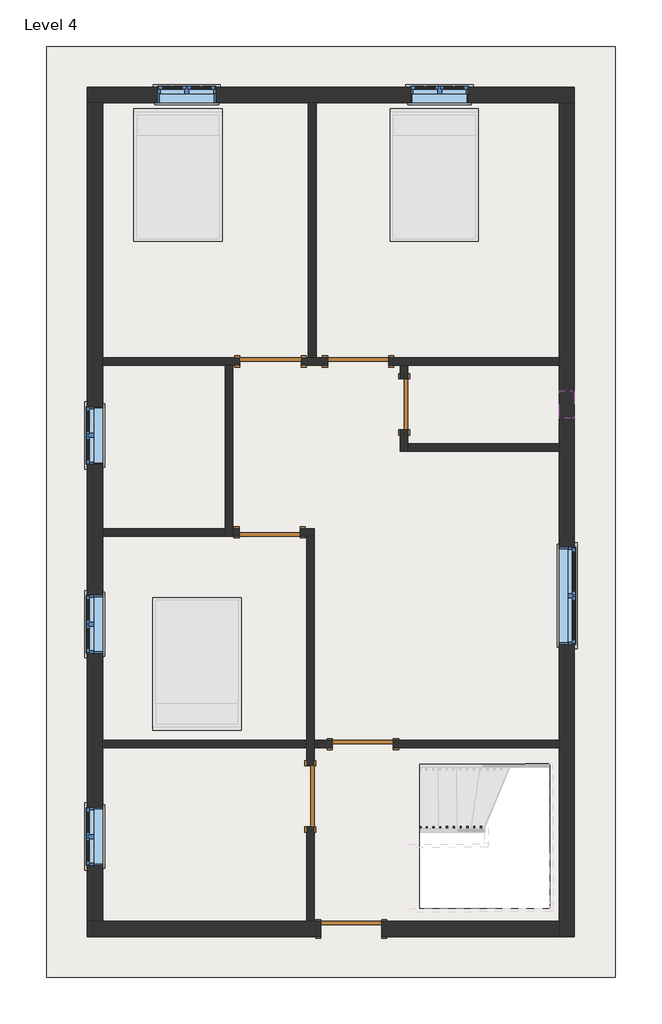
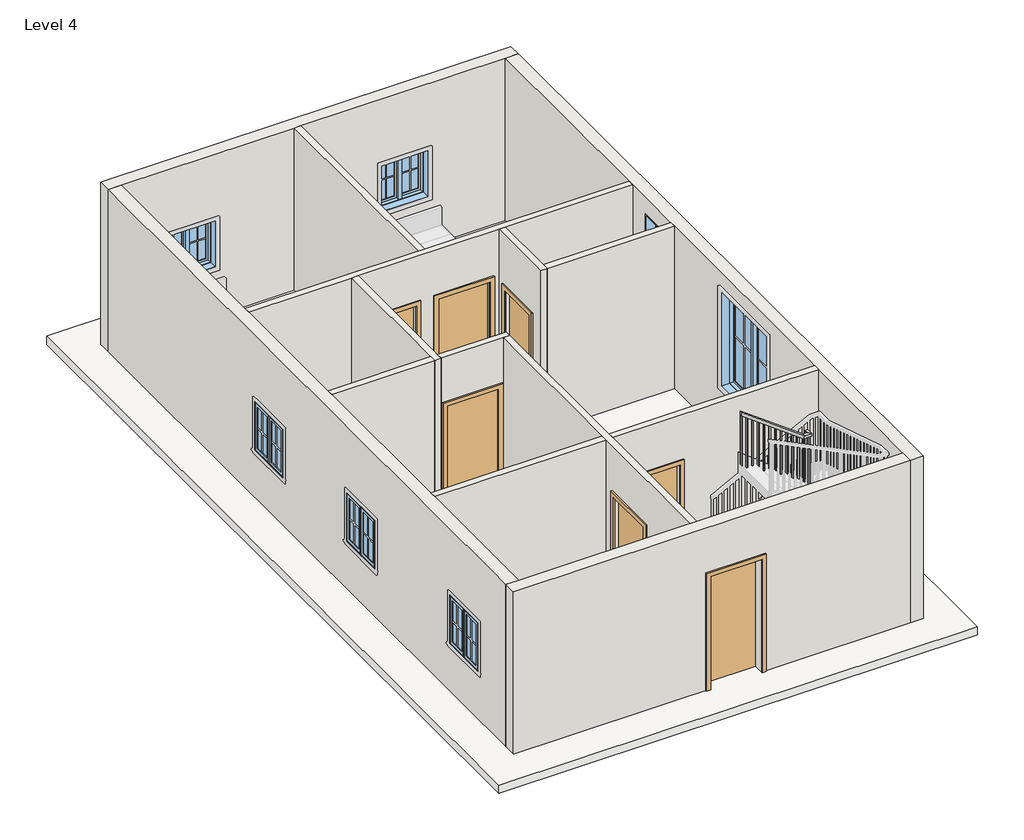
# One storey, part 1 of 2: 13 walls, 7 doors, 7 windows, 1 railing, 1 roof.
"""IFC4 building model written with IfcOpenShell, lengths in millimetres."""

from ifc_helpers import new_model, si_unit, frame, origin, place, context, project, spatial, polyline, outline, extrude, faceted_brep, transform, mapped, element, save
from components import door_f2b275c1, door_e5f9f3c4, door_305aa2a5, door_a90ba1ad, window_aa618e30, window_339605e1, window_9ac97e1a

model = new_model("IFC4")

# Units and contexts
model_context = context("Model", 3, world=origin())
ifc_project = project(units=[si_unit("LENGTHUNIT", "METRE", prefix="MILLI")], contexts=[model_context])

# Site, building, storey
site = spatial("IfcSite", under=ifc_project)
building = spatial("IfcBuilding", under=site)
storey = spatial("IfcBuildingStorey", under=building, Name="Level 4", Elevation=6400.8)

# Doors
placement = place(None, origin())
door_shape = door_f2b275c1(model_context)
element("IfcDoor", 1, ObjectType="Single-Flush : 30\" x 80\"", at=placement, inside=storey, context=model_context, shape_type="MappedRepresentation", body=[
    mapped(door_shape, transform((-163.0415084, 2144.7435985, 6400.8), x_axis=(0.0, 1.0, 0.0), y_axis=(-1.0, 0.0, 0.0), z_axis=(0.0, 0.0, 1.0))),
])
door_2_shape = door_e5f9f3c4(model_context)
element("IfcDoor", 2, ObjectType="Single-Flush : 36\" x 84\"", at=placement, inside=storey, context=model_context, shape_type="MappedRepresentation", body=[
    mapped(door_2_shape, transform((-2156.9415084, 2786.0935985, 6400.8), x_axis=(1.0, 0.0, 0.0), y_axis=(0.0, 1.0, 0.0), z_axis=(0.0, 0.0, 1.0))),
])
door_3_shape = door_305aa2a5(model_context)
element("IfcDoor", 3, ObjectType="Single-Flush : 36\" x 84\"", at=placement, inside=storey, context=model_context, shape_type="MappedRepresentation", body=[
    mapped(door_3_shape, transform((-848.8415084, 2786.0935985, 6400.8), x_axis=(-1.0, 0.0, 0.0), y_axis=(0.0, -1.0, 0.0), z_axis=(0.0, 0.0, 1.0))),
])
element("IfcDoor", 4, ObjectType="Single-Flush : 36\" x 84\"", at=placement, inside=storey, context=model_context, shape_type="MappedRepresentation", body=[
    mapped(door_3_shape, transform((-2170.1582019, 233.3935985, 6400.8), x_axis=(1.0, 0.0, 0.0), y_axis=(0.0, 1.0, 0.0), z_axis=(0.0, 0.0, 1.0))),
])
element("IfcDoor", 5, ObjectType="Single-Flush : 36\" x 84\"", at=placement, inside=storey, context=model_context, shape_type="MappedRepresentation", body=[
    mapped(door_3_shape, transform((-778.9915084, -2928.9064015, 6400.8), x_axis=(-1.0, 0.0, 0.0), y_axis=(0.0, -1.0, 0.0), z_axis=(0.0, 0.0, 1.0))),
])
element("IfcDoor", 6, ObjectType="Single-Flush : 36\" x 84\"", at=placement, inside=storey, context=model_context, shape_type="MappedRepresentation", body=[
    mapped(door_3_shape, transform((-1561.0748955, -3709.9564015, 6400.8), x_axis=(0.0, 1.0, 0.0), y_axis=(-1.0, 0.0, 0.0), z_axis=(0.0, 0.0, 1.0))),
])
door_4_shape = door_a90ba1ad(model_context)
element("IfcDoor", 7, ObjectType="Single-Flush : 36\" x 84\"", at=placement, inside=storey, context=model_context, shape_type="MappedRepresentation", body=[
    mapped(door_4_shape, transform((-951.4748955, -5691.1564015, 6400.8), x_axis=(-1.0, 0.0, 0.0), y_axis=(0.0, -1.0, 0.0), z_axis=(0.0, 0.0, 1.0))),
])

# Railing
element("IfcRailing", 8, ObjectType="Handrail - Rectangular", at=placement, inside=storey, context=model_context, shape_type="SolidModel", body=[
    faceted_brep([(73.2591805, -4146.3303197, 7992.5333333), (73.2591805, -4146.3303197, 7925.9495342), (73.5214139, -4197.1296428, 7925.9495342), (73.5214139, -4197.1296428, 7992.5333333), (1064.2769136, -4141.2145447, 8832.2511215), (1082.90463, -4141.1183857, 8781.4511215), (1083.1668634, -4191.9177089, 8781.4511215), (1064.5391469, -4192.0138678, 8832.2511215), (1144.655904, -4140.7996168, 8832.2511215), (1144.9181373, -4191.59894, 8832.2511215), (1144.9181373, -4191.59894, 8781.4511215), (1144.655904, -4140.7996168, 8781.4511215)], [[[0, 1, 2, 3]], [[1, 0, 4, 5]], [[2, 1, 5, 6]], [[3, 2, 6, 7]], [[0, 3, 7, 4]], [[8, 9, 10, 11]], [[5, 4, 8, 11]], [[6, 5, 11, 10]], [[7, 6, 10, 9]], [[4, 7, 9, 8]]]),
    faceted_brep([(1144.9181373, -4191.59894, 8840.7305642), (1144.9181373, -4191.59894, 8719.448826), (1094.1188142, -4191.8611734, 8719.448826), (1094.1188142, -4191.8611734, 8840.7305642), (1145.9670708, -4394.7962326, 9281.2506209), (1146.2293041, -4445.5955558, 9270.0988968), (1095.429981, -4445.8577892, 9270.0988968), (1095.1677476, -4395.058466, 9281.2506209), (1145.9670708, -4394.7962326, 9531.8424257), (1146.2293041, -4445.5955558, 9481.0424257), (1095.429981, -4445.8577892, 9481.0424257), (1095.1677476, -4395.058466, 9531.8424257), (1146.6226542, -4521.7945406, 9531.8424257), (1146.6226542, -4521.7945406, 9481.0424257), (1095.5610976, -4471.2574507, 9481.0424257), (1095.5610976, -4471.2574507, 9531.8424257), (1019.6243463, -4522.4501239, 9531.8424257), (1002.8333893, -4522.5368013, 9481.0424257), (1002.5711559, -4471.7374781, 9481.0424257), (1019.3621129, -4471.6508008, 9531.8424257), (-100.5579777, -4528.232665, 10363.2), (-100.8202111, -4477.4333418, 10363.2), (-100.8202111, -4477.4333418, 10299.9383775), (-100.5579777, -4528.232665, 10299.9383775)], [[[0, 1, 2, 3]], [[1, 0, 4, 5]], [[2, 1, 5, 6]], [[3, 2, 6, 7]], [[0, 3, 7, 4]], [[5, 4, 8, 9]], [[6, 5, 9, 10]], [[7, 6, 10, 11]], [[4, 7, 11, 8]], [[9, 8, 12, 13]], [[10, 9, 13, 14]], [[11, 10, 14, 15]], [[8, 11, 15, 12]], [[13, 12, 16, 17]], [[14, 13, 17, 18]], [[15, 14, 18, 19]], [[12, 15, 19, 16]], [[20, 21, 22, 23]], [[17, 16, 20, 23]], [[18, 17, 23, 22]], [[19, 18, 22, 21]], [[16, 19, 21, 20]]]),
    extrude(outline(polyline([(235.6690058, -19.05), (221.5309941, 0.0), (1247.144155, 0.0), (1247.144155, -19.05), (235.6690058, -19.05)])), frame((-107.5675843, -4512.3936381, 10526.6108217), z_axis=(-0.005162073969672187, 0.9999866764074069, 0.0), x_axis=(0.0, 0.0, -1.0)), (0.0, 0.0, 1.0), 19.05),
    extrude(outline(polyline([(235.6690059, -19.05), (221.5309942, 0.0), (1171.7414261, 0.0), (1171.7414261, -19.05), (235.6690059, -19.05)])), frame((-5.968938, -4511.8691714, 10451.2080928), z_axis=(-0.005162073969672187, 0.9999866764074069, 0.0), x_axis=(0.0, 0.0, -1.0)), (0.0, 0.0, 1.0), 19.05),
    extrude(outline(polyline([(235.6690058, -19.05), (221.5309941, 0.0), (1096.3386971, 0.0), (1096.3386971, -19.05), (235.6690058, -19.05)])), frame((95.6297083, -4511.3447046, 10375.8053638), z_axis=(-0.005162073969672187, 0.9999866764074069, 0.0), x_axis=(0.0, 0.0, -1.0)), (0.0, 0.0, 1.0), 19.05),
    extrude(outline(polyline([(235.6690059, -19.0499999), (221.5309942, 0.0), (1190.2693016, 0.0), (1190.2693016, -19.0499999), (235.6690059, -19.0499999)])), frame((197.2283547, -4510.8202379, 10300.4026349), z_axis=(-0.005162073969672187, 0.9999866764074069, 0.0), x_axis=(0.0, 0.0, -1.0)), (0.0, 0.0, 1.0), 19.05),
    extrude(outline(polyline([(235.6690058, -19.05), (221.5309942, 0.0), (1114.8665726, 0.0), (1114.8665726, -19.05), (235.6690058, -19.05)])), frame((298.827001, -4510.2957712, 10224.9999059), z_axis=(-0.005162073969672187, 0.9999866764074069, 0.0), x_axis=(0.0, 0.0, -1.0)), (0.0, 0.0, 1.0), 19.05),
    extrude(outline(polyline([(235.6690058, -19.05), (221.5309941, 0.0), (1039.4638436, 0.0), (1039.4638436, -19.05), (235.6690058, -19.05)])), frame((400.4256473, -4509.7713045, 10149.5971769), z_axis=(-0.005162073969672187, 0.9999866764074069, 0.0), x_axis=(0.0, 0.0, -1.0)), (0.0, 0.0, 1.0), 19.05),
    extrude(outline(polyline([(235.6690058, -19.05), (221.5309942, 0.0), (1133.394448, 0.0), (1133.394448, -19.05), (235.6690058, -19.05)])), frame((502.0242936, -4509.2468378, 10074.194448), z_axis=(-0.005162073969672187, 0.9999866764074069, 0.0), x_axis=(0.0, 0.0, -1.0)), (0.0, 0.0, 1.0), 19.05),
    extrude(outline(polyline([(235.6690058, -19.05), (221.5309941, 0.0), (1057.991719, 0.0), (1057.991719, -19.05), (235.6690058, -19.05)])), frame((603.6229399, -4508.7223711, 9998.791719), z_axis=(-0.005162073969672187, 0.9999866764074069, 0.0), x_axis=(0.0, 0.0, -1.0)), (0.0, 0.0, 1.0), 19.05),
    extrude(outline(polyline([(235.6690059, -19.05), (221.5309942, 0.0), (1151.9223234, 0.0), (1151.9223234, -19.05), (235.6690059, -19.05)])), frame((705.2215863, -4508.1979044, 9923.3889901), z_axis=(-0.005162073969672187, 0.9999866764074069, 0.0), x_axis=(0.0, 0.0, -1.0)), (0.0, 0.0, 1.0), 19.05),
    extrude(outline(polyline([(235.6690058, -19.05), (221.5309941, 0.0), (1076.5195944, 0.0), (1076.5195944, -19.05), (235.6690058, -19.05)])), frame((806.8202326, -4507.6734376, 9847.9862611), z_axis=(-0.005162073969672187, 0.9999866764074069, 0.0), x_axis=(0.0, 0.0, -1.0)), (0.0, 0.0, 1.0), 19.05),
    extrude(outline(polyline([(235.6690059, -19.05), (221.5309942, 0.0), (1170.4501989, 0.0), (1170.4501989, -19.05), (235.6690059, -19.05)])), frame((908.4188789, -4507.1489709, 9772.5835322), z_axis=(-0.005162073969672187, 0.9999866764074069, 0.0), x_axis=(0.0, 0.0, -1.0)), (0.0, 0.0, 1.0), 19.05),
    extrude(outline(polyline([(235.6690058, -19.05), (221.5309942, 0.0), (1095.0474699, 0.0), (1095.0474699, -19.05), (235.6690058, -19.05)])), frame((1010.0175252, -4506.6245042, 9697.1808032), z_axis=(-0.005162073969672187, 0.9999866764074069, 0.0), x_axis=(0.0, 0.0, -1.0)), (0.0, 0.0, 1.0), 19.05),
    extrude(outline(polyline([(1111.3867174, -4461.6506297), (1130.4364636, -4461.5522922), (1130.5348011, -4480.6020384), (1111.4850549, -4480.7003759), (1111.3867174, -4461.6506297)])), frame((0.0, 0.0, 8432.8), z_axis=(0.0, 0.0, 1.0), x_axis=(1.0, 0.0, 0.0)), (0.0, 0.0, 1.0), 1048.2424257),
    extrude(outline(polyline([(207.9506224, -19.05), (249.2493777, 0.0), (1070.0372089, 0.0), (1070.0372089, -19.05), (207.9506224, -19.05)])), frame((1110.8622507, -4360.0519834, 9333.5038756), z_axis=(0.9999866764074068, 0.005162073969671281, 0.0), x_axis=(0.0, 0.0, -1.0)), (0.0, 0.0, 1.0), 19.05),
    extrude(outline(polyline([(207.9506224, -19.05), (249.2493777, 0.0), (1019.110514, 0.0), (1019.110514, -19.05), (207.9506224, -19.05)])), frame((1110.3377839, -4258.4533371, 9113.2438473), z_axis=(0.9999866764074068, 0.005162073969671281, 0.0), x_axis=(0.0, 0.0, -1.0)), (0.0, 0.0, 1.0), 19.05),
    extrude(outline(polyline([(1079.9010561, -4176.0593559), (1079.8027186, -4157.0096098), (1098.8524648, -4156.9112722), (1098.9508023, -4175.9610184), (1079.9010561, -4176.0593559)])), frame((0.0, 0.0, 7755.4666667), z_axis=(0.0, 0.0, 1.0), x_axis=(1.0, 0.0, 0.0)), (0.0, 0.0, 1.0), 1025.9844548),
    extrude(outline(polyline([(220.5293015, -19.05), (236.6706986, 0.0), (1343.2032603, 0.0), (1343.2032603, -19.05), (220.5293015, -19.05)])), frame((978.3024098, -4176.5838227, 8929.3365936), z_axis=(-0.005162073969671482, 0.9999866764074068, 0.0), x_axis=(0.0, 0.0, -1.0)), (0.0, 0.0, 1.0), 19.05),
    extrude(outline(polyline([(220.5293015, -19.05), (236.6706985, 0.0), (1257.1158092, 0.0), (1257.1158092, -19.05), (220.5293015, -19.05)])), frame((876.7037635, -4177.1082894, 8843.2491425), z_axis=(-0.005162073969671482, 0.9999866764074068, 0.0), x_axis=(0.0, 0.0, -1.0)), (0.0, 0.0, 1.0), 19.05),
    extrude(outline(polyline([(220.5293015, -19.05), (236.6706986, 0.0), (1340.3616915, 0.0), (1340.3616915, -19.05), (220.5293015, -19.05)])), frame((775.1051171, -4177.6327561, 8757.1616915), z_axis=(-0.005162073969671482, 0.9999866764074068, 0.0), x_axis=(0.0, 0.0, -1.0)), (0.0, 0.0, 1.0), 19.05),
    extrude(outline(polyline([(220.5293014, -19.05), (236.6706985, 0.0), (1254.2742404, 0.0), (1254.2742404, -19.05), (220.5293014, -19.05)])), frame((673.5064708, -4178.1572228, 8671.0742404), z_axis=(-0.005162073969671482, 0.9999866764074068, 0.0), x_axis=(0.0, 0.0, -1.0)), (0.0, 0.0, 1.0), 19.05),
    extrude(outline(polyline([(220.5293015, -19.05), (236.6706985, 0.0), (1337.5201227, 0.0), (1337.5201227, -19.05), (220.5293015, -19.05)])), frame((571.9078245, -4178.6816895, 8584.9867894), z_axis=(-0.005162073969671482, 0.9999866764074068, 0.0), x_axis=(0.0, 0.0, -1.0)), (0.0, 0.0, 1.0), 19.05),
    extrude(outline(polyline([(220.5293015, -19.05), (236.6706986, 0.0), (1251.4326717, 0.0), (1251.4326717, -19.05), (220.5293015, -19.05)])), frame((470.3091782, -4179.2061562, 8498.8993384), z_axis=(-0.005162073969671482, 0.9999866764074068, 0.0), x_axis=(0.0, 0.0, -1.0)), (0.0, 0.0, 1.0), 19.05),
    extrude(outline(polyline([(220.5293014, -19.0499999), (236.6706985, 0.0), (1165.3452206, 0.0), (1165.3452206, -19.0499999), (220.5293014, -19.0499999)])), frame((368.7105319, -4179.7306229, 8412.8118873), z_axis=(-0.005162073969671482, 0.9999866764074068, 0.0), x_axis=(0.0, 0.0, -1.0)), (0.0, 0.0, 1.0), 19.05),
    extrude(outline(polyline([(220.5293015, -19.05), (236.6706986, 0.0), (1248.591103, 0.0), (1248.591103, -19.05), (220.5293015, -19.05)])), frame((267.1118855, -4180.2550897, 8326.7244363), z_axis=(-0.005162073969671482, 0.9999866764074068, 0.0), x_axis=(0.0, 0.0, -1.0)), (0.0, 0.0, 1.0), 19.05),
    extrude(outline(polyline([(220.5293014, -19.05), (236.6706985, 0.0), (1162.5036519, 0.0), (1162.5036519, -19.05), (220.5293014, -19.05)])), frame((165.5132392, -4180.7795564, 8240.6369852), z_axis=(-0.005162073969671482, 0.9999866764074068, 0.0), x_axis=(0.0, 0.0, -1.0)), (0.0, 0.0, 1.0), 19.05),
    extrude(outline(polyline([(1111.5178341, -4487.0502913), (1130.5675802, -4486.9519538), (1130.6659177, -4506.0017), (1111.6161716, -4506.1000375), (1111.5178341, -4487.0502913)])), frame((0.0, 0.0, 8432.8), z_axis=(0.0, 0.0, 1.0), x_axis=(1.0, 0.0, 0.0)), (0.0, 0.0, 1.0), 1048.2424257),
    extrude(outline(polyline([(1109.9116547, -4175.9044369), (1109.8133172, -4156.8546908), (1128.8630634, -4156.7563533), (1128.9614009, -4175.8060994), (1109.9116547, -4175.9044369)])), frame((0.0, 0.0, 7924.8), z_axis=(0.0, 0.0, 1.0), x_axis=(1.0, 0.0, 0.0)), (0.0, 0.0, 1.0), 856.6511215),
    extrude(outline(polyline([(235.6690058, -19.05), (221.5309941, 0.0), (1242.0027049, 0.0), (1242.0027049, -19.05), (235.6690058, -19.05)])), frame((-100.6399256, -4512.3578765, 10521.4693716), z_axis=(-0.005162073969672187, 0.9999866764074069, 0.0), x_axis=(0.0, 0.0, -1.0)), (0.0, 0.0, 1.0), 19.05),
    extrude(outline(polyline([(220.5293014, -19.05), (236.6706985, 0.0), (1084.4868994, 0.0), (1084.4868994, -19.05), (220.5293014, -19.05)])), frame((73.439466, -4181.2548543, 8162.6202327), z_axis=(-0.005162073969671482, 0.9999866764074068, 0.0), x_axis=(0.0, 0.0, -1.0)), (0.0, 0.0, 1.0), 19.05),
])

# Roof
element("IfcRoof", 9, ObjectType="Generic - 12\"", at=placement, inside=storey, context=model_context, shape_type="SweptSolid", body=[
    extrude(outline(polyline([(-5503.3915084, -6415.0564015), (-5503.3915084, 7491.4435985), (2992.9084916, 7491.4435985), (2992.9084916, -6415.0564015), (-5503.3915084, -6415.0564015)]), holes=[polyline([(2014.669115, -3231.9425028), (68.5389801, -3231.9425028), (68.5389801, -5380.9250672), (2014.669115, -5380.9250672), (2014.669115, -3231.9425028)])]), frame((0.0, 0.0, 6248.4), z_axis=(0.0, 0.0, 1.0), x_axis=(1.0, 0.0, 0.0)), (0.0, 0.0, 1.0), 152.4),
])

# Walls
element("IfcWall", 10, ObjectType="WALL4.5\"", at=placement, inside=storey, context=model_context, shape_type="Brep", body=[
    faceted_brep([(-1699.7415084, 2728.9435985, 6400.8), (-1306.0415084, 2728.9435985, 6400.8), (-1306.0415084, 2728.9435985, 8534.4), (-391.6415084, 2728.9435985, 8534.4), (-391.6415084, 2728.9435985, 6400.8), (-220.1915084, 2728.9435985, 6400.8), (-105.8915084, 2728.9435985, 6400.8), (2154.7084916, 2728.9435985, 6400.8), (2154.7084916, 2728.9435985, 9448.8), (-105.8915084, 2728.9435985, 9448.8), (-220.1915084, 2728.9435985, 9448.8), (-2722.0915084, 2728.9435985, 9448.8), (-2836.3915084, 2728.9435985, 9448.8), (-4665.1915084, 2728.9435985, 9448.8), (-4665.1915084, 2728.9435985, 6400.8), (-2836.3915084, 2728.9435985, 6400.8), (-2722.0915084, 2728.9435985, 6400.8), (-2614.1415084, 2728.9435985, 6400.8), (-2614.1415084, 2728.9435985, 8534.4), (-1699.7415084, 2728.9435985, 8534.4), (-1306.0415084, 2843.2435985, 8534.4), (-1306.0415084, 2843.2435985, 6400.8), (-1477.4915084, 2843.2435985, 6400.8), (-1591.7915084, 2843.2435985, 6400.8), (-1699.7415084, 2843.2435985, 6400.8), (-1699.7415084, 2843.2435985, 8534.4), (-2614.1415084, 2843.2435985, 8534.4), (-2614.1415084, 2843.2435985, 6400.8), (-4665.1915084, 2843.2435985, 6400.8), (-4665.1915084, 2843.2435985, 9448.8), (-1591.7915084, 2843.2435985, 9448.8), (-1477.4915084, 2843.2435985, 9448.8), (2154.7084916, 2843.2435985, 9448.8), (2154.7084916, 2843.2435985, 6400.8), (-391.6415084, 2843.2435985, 6400.8), (-391.6415084, 2843.2435985, 8534.4)], [[[0, 1, 2, 3, 4, 5, 6, 7, 8, 9, 10, 11, 12, 13, 14, 15, 16, 17, 18, 19]], [[20, 21, 22, 23, 24, 25, 26, 27, 28, 29, 30, 31, 32, 33, 34, 35]], [[17, 16, 15, 14, 28, 27]], [[34, 33, 7, 6, 5, 4]], [[24, 23, 22, 21, 1, 0]], [[8, 7, 33, 32]], [[14, 13, 29, 28]], [[25, 24, 0, 19]], [[26, 25, 19, 18]], [[27, 26, 18, 17]], [[2, 1, 21, 20]], [[3, 2, 20, 35]], [[4, 3, 35, 34]], [[13, 12, 11, 10, 9, 8, 32, 31, 30, 29]]]),
])
element("IfcWall", 11, ObjectType="WALL4.5\"", at=placement, inside=storey, context=model_context, shape_type="SweptSolid", body=[
    extrude(outline(polyline([(-1591.7915084, 2843.2435985), (-1591.7915084, 6653.2435985), (-1477.4915084, 6653.2435985), (-1477.4915084, 2843.2435985), (-1591.7915084, 2843.2435985)])), frame((0.0, 0.0, 6400.8), z_axis=(0.0, 0.0, 1.0), x_axis=(1.0, 0.0, 0.0)), (0.0, 0.0, 1.0), 3048.0),
])
element("IfcWall", 12, ObjectType="WALL4.5\"", at=placement, inside=storey, context=model_context, shape_type="Brep", body=[
    faceted_brep([(-2836.3915084, 2728.9435985, 6400.8), (-2836.3915084, 290.5435985, 6400.8), (-2836.3915084, 176.2435985, 6400.8), (-2836.3915084, 176.2435985, 9448.8), (-2836.3915084, 290.5435985, 9448.8), (-2836.3915084, 2728.9435985, 9448.8), (-2722.0915084, 2728.9435985, 6400.8), (-2722.0915084, 2728.9435985, 9448.8), (-2722.0915084, 290.5435985, 9448.8), (-2722.0915084, 176.2435985, 9448.8), (-2722.0915084, 176.2435985, 6400.8), (-2722.0915084, 290.5435985, 6400.8)], [[[0, 1, 2, 3, 4, 5]], [[6, 7, 8, 9, 10, 11]], [[2, 1, 0, 6, 11, 10]], [[0, 5, 7, 6]], [[3, 2, 10, 9]], [[5, 4, 3, 9, 8, 7]]]),
])
element("IfcWall", 13, ObjectType="WALL4.5\"", at=placement, inside=storey, context=model_context, shape_type="SweptSolid", body=[
    extrude(outline(polyline([(-2836.3915084, 176.2435985), (-4665.1915084, 176.2435985), (-4665.1915084, 290.5435985), (-2836.3915084, 290.5435985), (-2836.3915084, 176.2435985)])), frame((0.0, 0.0, 6400.8), z_axis=(0.0, 0.0, 1.0), x_axis=(1.0, 0.0, 0.0)), (0.0, 0.0, 1.0), 3048.0),
])
element("IfcWall", 14, ObjectType="WALL4.5\"", at=placement, inside=storey, context=model_context, shape_type="Brep", body=[
    faceted_brep([(-1712.9582019, 176.2435985, 8534.4), (-1712.9582019, 176.2435985, 6400.8), (-1618.2248955, 176.2435985, 6400.8), (-1503.9248955, 176.2435985, 6400.8), (-1502.8915084, 176.2435985, 6400.8), (-1502.8915084, 176.2435985, 9448.8), (-1503.9248955, 176.2435985, 9448.8), (-1618.2248955, 176.2435985, 9448.8), (-2722.0915084, 176.2435985, 9448.8), (-2722.0915084, 176.2435985, 6400.8), (-2627.3582019, 176.2435985, 6400.8), (-2627.3582019, 176.2435985, 8534.4), (-1502.8915084, 290.5435985, 6400.8), (-1712.9582019, 290.5435985, 6400.8), (-1712.9582019, 290.5435985, 8534.4), (-2627.3582019, 290.5435985, 8534.4), (-2627.3582019, 290.5435985, 6400.8), (-2722.0915084, 290.5435985, 6400.8), (-2722.0915084, 290.5435985, 9448.8), (-1502.8915084, 290.5435985, 9448.8)], [[[0, 1, 2, 3, 4, 5, 6, 7, 8, 9, 10, 11]], [[12, 13, 14, 15, 16, 17, 18, 19]], [[10, 9, 17, 16]], [[4, 3, 2, 1, 13, 12]], [[5, 4, 12, 19]], [[9, 8, 18, 17]], [[14, 13, 1, 0]], [[15, 14, 0, 11]], [[16, 15, 11, 10]], [[8, 7, 6, 5, 19, 18]]]),
])
element("IfcWall", 15, ObjectType="WALL4.5\"", at=placement, inside=storey, context=model_context, shape_type="Brep", body=[
    faceted_brep([(-1618.2248955, 176.2435985, 6400.8), (-1618.2248955, -2871.7564015, 6400.8), (-1618.2248955, -2986.0564015, 6400.8), (-1618.2248955, -3252.7564015, 6400.8), (-1618.2248955, -3252.7564015, 8534.4), (-1618.2248955, -4167.1564015, 8534.4), (-1618.2248955, -4167.1564015, 6400.8), (-1618.2248955, -5576.8564015, 6400.8), (-1618.2248955, -5576.8564015, 9448.8), (-1618.2248955, -2986.0564015, 9448.8), (-1618.2248955, -2871.7564015, 9448.8), (-1618.2248955, 176.2435985, 9448.8), (-1503.9248955, -3252.7564015, 8534.4), (-1503.9248955, -3252.7564015, 6400.8), (-1503.9248955, -2986.0564015, 6400.8), (-1503.9248955, -2871.7564015, 6400.8), (-1503.9248955, 176.2435985, 6400.8), (-1503.9248955, 176.2435985, 9448.8), (-1503.9248955, -2871.7564015, 9448.8), (-1503.9248955, -2986.0564015, 9448.8), (-1503.9248955, -5576.8564015, 9448.8), (-1503.9248955, -5576.8564015, 6400.8), (-1503.9248955, -4167.1564015, 6400.8), (-1503.9248955, -4167.1564015, 8534.4)], [[[0, 1, 2, 3, 4, 5, 6, 7, 8, 9, 10, 11]], [[12, 13, 14, 15, 16, 17, 18, 19, 20, 21, 22, 23]], [[22, 21, 7, 6]], [[16, 15, 14, 13, 3, 2, 1, 0]], [[8, 7, 21, 20]], [[0, 11, 17, 16]], [[4, 3, 13, 12]], [[5, 4, 12, 23]], [[6, 5, 23, 22]], [[11, 10, 9, 8, 20, 19, 18, 17]]]),
])
element("IfcWall", 16, ObjectType="WALL4.5\"", at=placement, inside=storey, context=model_context, shape_type="SweptSolid", body=[
    extrude(outline(polyline([(6400.8, 2154.7084916), (9448.8, 2154.7084916), (9448.8, -1503.9248955), (6400.8, -1503.9248955), (6400.8, -1236.1915084), (8534.4, -1236.1915084), (8534.4, -321.7915084), (6400.8, -321.7915084), (6400.8, 2154.7084916)])), frame((0.0, -2986.0564015, 0.0), z_axis=(0.0, 1.0, 0.0), x_axis=(0.0, 0.0, 1.0)), (0.0, 0.0, 1.0), 114.3),
    extrude(outline(polyline([(-4665.1915084, -2986.0564015), (-4665.1915084, -2871.7564015), (-1618.2248955, -2871.7564015), (-1618.2248955, -2986.0564015), (-4665.1915084, -2986.0564015)])), frame((0.0, 0.0, 6400.8), z_axis=(0.0, 0.0, 1.0), x_axis=(1.0, 0.0, 0.0)), (0.0, 0.0, 1.0), 3048.0),
])
element("IfcWall", 17, ObjectType="WALL4.5\"", at=placement, inside=storey, context=model_context, shape_type="Brep", body=[
    faceted_brep([(-220.1915084, 2728.9435985, 6400.8), (-220.1915084, 2525.7435985, 6400.8), (-220.1915084, 2525.7435985, 8432.8), (-220.1915084, 1763.7435985, 8432.8), (-220.1915084, 1763.7435985, 6400.8), (-220.1915084, 1446.2435985, 6400.8), (-220.1915084, 1446.2435985, 9448.8), (-220.1915084, 2728.9435985, 9448.8), (-105.8915084, 2525.7435985, 8432.8), (-105.8915084, 2525.7435985, 6400.8), (-105.8915084, 2728.9435985, 6400.8), (-105.8915084, 2728.9435985, 9448.8), (-105.8915084, 1560.5435985, 9448.8), (-105.8915084, 1446.2435985, 9448.8), (-105.8915084, 1446.2435985, 6400.8), (-105.8915084, 1560.5435985, 6400.8), (-105.8915084, 1763.7435985, 6400.8), (-105.8915084, 1763.7435985, 8432.8)], [[[0, 1, 2, 3, 4, 5, 6, 7]], [[8, 9, 10, 11, 12, 13, 14, 15, 16, 17]], [[10, 9, 1, 0]], [[16, 15, 14, 5, 4]], [[0, 7, 11, 10]], [[6, 5, 14, 13]], [[2, 1, 9, 8]], [[3, 2, 8, 17]], [[4, 3, 17, 16]], [[7, 6, 13, 12, 11]]]),
])
element("IfcWall", 18, ObjectType="WALL4.5\"", at=placement, inside=storey, context=model_context, shape_type="SweptSolid", body=[
    extrude(outline(polyline([(2154.7084916, 1446.2435985), (-105.8915084, 1446.2435985), (-105.8915084, 1560.5435985), (2154.7084916, 1560.5435985), (2154.7084916, 1446.2435985)])), frame((0.0, 0.0, 6400.8), z_axis=(0.0, 0.0, 1.0), x_axis=(1.0, 0.0, 0.0)), (0.0, 0.0, 1.0), 3048.0),
])
element("IfcWall", 19, ObjectType="WALL9\"", at=placement, inside=storey, context=model_context, shape_type="Brep", body=[
    faceted_brep([(-4893.7915084, 6653.2435985, 6400.8), (-4665.1915084, 6653.2435985, 6400.8), (-1591.7915084, 6653.2435985, 6400.8), (-1477.4915084, 6653.2435985, 6400.8), (2154.7084916, 6653.2435985, 6400.8), (2383.3084916, 6653.2435985, 6400.8), (2383.3084916, 6653.2435985, 9448.8), (2154.7084916, 6653.2435985, 9448.8), (-1477.4915084, 6653.2435985, 9448.8), (-1591.7915084, 6653.2435985, 9448.8), (-4665.1915084, 6653.2435985, 9448.8), (-4893.7915084, 6653.2435985, 9448.8), (-2976.0915084, 6653.2435985, 8229.6), (-2976.0915084, 6653.2435985, 7315.2), (-3839.6915084, 6653.2435985, 7315.2), (-3839.6915084, 6653.2435985, 8229.6), (798.9834916, 6653.2435985, 8229.6), (798.9834916, 6653.2435985, 7315.2), (-64.6165084, 6653.2435985, 7315.2), (-64.6165084, 6653.2435985, 8229.6), (-4893.7915084, 6881.8435985, 6400.8), (-4893.7915084, 6881.8435985, 9448.8), (2383.3084916, 6881.8435985, 9448.8), (2383.3084916, 6881.8435985, 6400.8), (-2976.0915084, 6881.8435985, 8229.6), (-3839.6915084, 6881.8435985, 8229.6), (-3839.6915084, 6881.8435985, 7315.2), (-2976.0915084, 6881.8435985, 7315.2), (798.9834916, 6881.8435985, 8229.6), (-64.6165084, 6881.8435985, 8229.6), (-64.6165084, 6881.8435985, 7315.2), (798.9834916, 6881.8435985, 7315.2)], [[[0, 1, 2, 3, 4, 5, 6, 7, 8, 9, 10, 11], [12, 13, 14, 15], [16, 17, 18, 19]], [[20, 21, 22, 23], [24, 25, 26, 27], [28, 29, 30, 31]], [[5, 4, 3, 2, 1, 0, 20, 23]], [[6, 5, 23, 22]], [[0, 11, 21, 20]], [[13, 12, 24, 27]], [[14, 13, 27, 26]], [[15, 14, 26, 25]], [[12, 15, 25, 24]], [[17, 16, 28, 31]], [[18, 17, 31, 30]], [[19, 18, 30, 29]], [[16, 19, 29, 28]], [[11, 10, 9, 8, 7, 6, 22, 21]]]),
])
element("IfcWall", 20, ObjectType="WALL9\"", at=placement, inside=storey, context=model_context, shape_type="Brep", body=[
    faceted_brep([(2154.7084916, 6653.2435985, 6400.8), (2154.7084916, 2843.2435985, 6400.8), (2154.7084916, 2728.9435985, 6400.8), (2154.7084916, 1560.5435985, 6400.8), (2154.7084916, 1446.2435985, 6400.8), (2154.7084916, -2871.7564015, 6400.8), (2154.7084916, -2986.0564015, 6400.8), (2154.7084916, -5576.8564015, 6400.8), (2154.7084916, -5805.4564015, 6400.8), (2154.7084916, -5805.4564015, 9448.8), (2154.7084916, -5576.8564015, 9448.8), (2154.7084916, -2986.0564015, 9448.8), (2154.7084916, -2871.7564015, 9448.8), (2154.7084916, 1446.2435985, 9448.8), (2154.7084916, 1560.5435985, 9448.8), (2154.7084916, 2728.9435985, 9448.8), (2154.7084916, 2843.2435985, 9448.8), (2154.7084916, 6653.2435985, 9448.8), (2154.7084916, 1941.5435985, 9144.0), (2154.7084916, 1941.5435985, 8534.4), (2154.7084916, 2347.9435985, 8534.4), (2154.7084916, 2347.9435985, 9144.0), (2154.7084916, -1436.6564015, 9144.0), (2154.7084916, -1436.6564015, 7315.2), (2154.7084916, 11.1435985, 7315.2), (2154.7084916, 11.1435985, 9144.0), (2383.3084916, 6653.2435985, 6400.8), (2383.3084916, 6653.2435985, 9448.8), (2383.3084916, -5805.4564015, 9448.8), (2383.3084916, -5805.4564015, 6400.8), (2383.3084916, 1941.5435985, 9144.0), (2383.3084916, 2347.9435985, 9144.0), (2383.3084916, 2347.9435985, 8534.4), (2383.3084916, 1941.5435985, 8534.4), (2383.3084916, -1436.6564015, 9144.0), (2383.3084916, 11.1435985, 9144.0), (2383.3084916, 11.1435985, 7315.2), (2383.3084916, -1436.6564015, 7315.2)], [[[0, 1, 2, 3, 4, 5, 6, 7, 8, 9, 10, 11, 12, 13, 14, 15, 16, 17], [18, 19, 20, 21], [22, 23, 24, 25]], [[26, 27, 28, 29], [30, 31, 32, 33], [34, 35, 36, 37]], [[8, 7, 6, 5, 4, 3, 2, 1, 0, 26, 29]], [[0, 17, 27, 26]], [[9, 8, 29, 28]], [[19, 18, 30, 33]], [[20, 19, 33, 32]], [[21, 20, 32, 31]], [[18, 21, 31, 30]], [[23, 22, 34, 37]], [[24, 23, 37, 36]], [[25, 24, 36, 35]], [[22, 25, 35, 34]], [[17, 16, 15, 14, 13, 12, 11, 10, 9, 28, 27]]]),
])
element("IfcWall", 21, ObjectType="WALL9\"", at=placement, inside=storey, context=model_context, shape_type="Brep", body=[
    faceted_brep([(-1408.6748955, -5576.8564015, 8534.4), (-1408.6748955, -5576.8564015, 6400.8), (-1503.9248955, -5576.8564015, 6400.8), (-1618.2248955, -5576.8564015, 6400.8), (-4665.1915084, -5576.8564015, 6400.8), (-4893.7915084, -5576.8564015, 6400.8), (-4893.7915084, -5576.8564015, 9448.8), (-4665.1915084, -5576.8564015, 9448.8), (-1618.2248955, -5576.8564015, 9448.8), (-1503.9248955, -5576.8564015, 9448.8), (2154.7084916, -5576.8564015, 9448.8), (2154.7084916, -5576.8564015, 6400.8), (-494.2748955, -5576.8564015, 6400.8), (-494.2748955, -5576.8564015, 8534.4), (-4893.7915084, -5805.4564015, 6400.8), (-1408.6748955, -5805.4564015, 6400.8), (-1408.6748955, -5805.4564015, 8534.4), (-494.2748955, -5805.4564015, 8534.4), (-494.2748955, -5805.4564015, 6400.8), (2154.7084916, -5805.4564015, 6400.8), (2154.7084916, -5805.4564015, 9448.8), (-4893.7915084, -5805.4564015, 9448.8)], [[[0, 1, 2, 3, 4, 5, 6, 7, 8, 9, 10, 11, 12, 13]], [[14, 15, 16, 17, 18, 19, 20, 21]], [[12, 11, 19, 18]], [[5, 4, 3, 2, 1, 15, 14]], [[11, 10, 20, 19]], [[6, 5, 14, 21]], [[16, 15, 1, 0]], [[17, 16, 0, 13]], [[18, 17, 13, 12]], [[10, 9, 8, 7, 6, 21, 20]]]),
])
element("IfcWall", 22, ObjectType="WALL9\"", at=placement, inside=storey, context=model_context, shape_type="Brep", body=[
    faceted_brep([(-4665.1915084, -5576.8564015, 6400.8), (-4665.1915084, -2986.0564015, 6400.8), (-4665.1915084, -2871.7564015, 6400.8), (-4665.1915084, 176.2435985, 6400.8), (-4665.1915084, 290.5435985, 6400.8), (-4665.1915084, 2728.9435985, 6400.8), (-4665.1915084, 2843.2435985, 6400.8), (-4665.1915084, 6653.2435985, 6400.8), (-4665.1915084, 6653.2435985, 9448.8), (-4665.1915084, 2843.2435985, 9448.8), (-4665.1915084, 2728.9435985, 9448.8), (-4665.1915084, 290.5435985, 9448.8), (-4665.1915084, 176.2435985, 9448.8), (-4665.1915084, -2871.7564015, 9448.8), (-4665.1915084, -2986.0564015, 9448.8), (-4665.1915084, -5576.8564015, 9448.8), (-4665.1915084, 2112.9935985, 8229.6), (-4665.1915084, 2112.9935985, 7315.2), (-4665.1915084, 1249.3935985, 7315.2), (-4665.1915084, 1249.3935985, 8229.6), (-4665.1915084, -706.4064015, 8229.6), (-4665.1915084, -706.4064015, 7315.2), (-4665.1915084, -1570.0064015, 7315.2), (-4665.1915084, -1570.0064015, 8229.6), (-4665.1915084, -3878.2314015, 8229.6), (-4665.1915084, -3878.2314015, 7315.2), (-4665.1915084, -4741.8314015, 7315.2), (-4665.1915084, -4741.8314015, 8229.6), (-4893.7915084, -5576.8564015, 6400.8), (-4893.7915084, -5576.8564015, 9448.8), (-4893.7915084, 6653.2435985, 9448.8), (-4893.7915084, 6653.2435985, 6400.8), (-4893.7915084, 2112.9935985, 8229.6), (-4893.7915084, 1249.3935985, 8229.6), (-4893.7915084, 1249.3935985, 7315.2), (-4893.7915084, 2112.9935985, 7315.2), (-4893.7915084, -706.4064015, 8229.6), (-4893.7915084, -1570.0064015, 8229.6), (-4893.7915084, -1570.0064015, 7315.2), (-4893.7915084, -706.4064015, 7315.2), (-4893.7915084, -3878.2314015, 8229.6), (-4893.7915084, -4741.8314015, 8229.6), (-4893.7915084, -4741.8314015, 7315.2), (-4893.7915084, -3878.2314015, 7315.2)], [[[0, 1, 2, 3, 4, 5, 6, 7, 8, 9, 10, 11, 12, 13, 14, 15], [16, 17, 18, 19], [20, 21, 22, 23], [24, 25, 26, 27]], [[28, 29, 30, 31], [32, 33, 34, 35], [36, 37, 38, 39], [40, 41, 42, 43]], [[7, 6, 5, 4, 3, 2, 1, 0, 28, 31]], [[0, 15, 29, 28]], [[8, 7, 31, 30]], [[17, 16, 32, 35]], [[18, 17, 35, 34]], [[19, 18, 34, 33]], [[16, 19, 33, 32]], [[21, 20, 36, 39]], [[22, 21, 39, 38]], [[23, 22, 38, 37]], [[20, 23, 37, 36]], [[25, 24, 40, 43]], [[26, 25, 43, 42]], [[27, 26, 42, 41]], [[24, 27, 41, 40]], [[15, 14, 13, 12, 11, 10, 9, 8, 30, 29]]]),
])

# Windows
window_shape = window_aa618e30(model_context)
element("IfcWindow", 23, ObjectType="Fixed : 16\" x 24\"", at=placement, inside=storey, context=model_context, shape_type="MappedRepresentation", body=[
    mapped(window_shape, transform((2269.0084916, 2106.6435985, 7620.0), x_axis=(0.0, -1.0, 0.0), y_axis=(1.0, 0.0, 0.0), z_axis=(0.0, 0.0, 1.0))),
])
window_2_shape = window_339605e1(model_context)
element("IfcWindow", 24, ObjectType="Window-Casement-Double : 34\" x 36\"", at=placement, inside=storey, context=model_context, shape_type="MappedRepresentation", body=[
    mapped(window_2_shape, transform((-3407.8915084, 6767.5435985, 6400.8), x_axis=(1.0, 0.0, 0.0), y_axis=(0.0, 1.0, 0.0), z_axis=(0.0, 0.0, 1.0))),
])
element("IfcWindow", 25, ObjectType="Window-Casement-Double : 34\" x 36\"", at=placement, inside=storey, context=model_context, shape_type="MappedRepresentation", body=[
    mapped(window_2_shape, transform((367.1834916, 6767.5435985, 6400.8), x_axis=(1.0, 0.0, 0.0), y_axis=(0.0, 1.0, 0.0), z_axis=(0.0, 0.0, 1.0))),
])
element("IfcWindow", 26, ObjectType="Window-Casement-Double : 34\" x 36\"", at=placement, inside=storey, context=model_context, shape_type="MappedRepresentation", body=[
    mapped(window_2_shape, transform((-4779.4915084, 1681.1935985, 6400.8), x_axis=(0.0, 1.0, 0.0), y_axis=(-1.0, 0.0, 0.0), z_axis=(0.0, 0.0, 1.0))),
])
element("IfcWindow", 27, ObjectType="Window-Casement-Double : 34\" x 36\"", at=placement, inside=storey, context=model_context, shape_type="MappedRepresentation", body=[
    mapped(window_2_shape, transform((-4779.4915084, -1138.2064015, 6400.8), x_axis=(0.0, 1.0, 0.0), y_axis=(-1.0, 0.0, 0.0), z_axis=(0.0, 0.0, 1.0))),
])
element("IfcWindow", 28, ObjectType="Window-Casement-Double : 34\" x 36\"", at=placement, inside=storey, context=model_context, shape_type="MappedRepresentation", body=[
    mapped(window_2_shape, transform((-4779.4915084, -4310.0314015, 6400.8), x_axis=(0.0, 1.0, 0.0), y_axis=(-1.0, 0.0, 0.0), z_axis=(0.0, 0.0, 1.0))),
])
window_3_shape = window_9ac97e1a(model_context)
element("IfcWindow", 29, ObjectType="Window-Casement-Double : 57\" x 72\"", at=placement, inside=storey, context=model_context, shape_type="MappedRepresentation", body=[
    mapped(window_3_shape, transform((2269.0084916, -712.7564015, 6400.8), x_axis=(0.0, -1.0, 0.0), y_axis=(1.0, 0.0, 0.0), z_axis=(0.0, 0.0, 1.0))),
])

save(model, "model.ifc")

# Revit data of these elements
# Type "Single-Flush : 30\" x 80\""
#   Type Mark = "5"
#   Construction Type Id = "MDOOR"
#   Assembly Code = "C1020"
#   Analytic Construction = "Metal"
#   Thickness = 0' - 2"
#   Heat Transfer Coefficient (U) = 0.651978 BTU/(h·ft²·°F)
#   Height = 6' - 8"
#   Trim Projection Ext = 0' - 1"
#   Trim Projection Int = 0' - 1"
#   Trim Width = 0' - 3"
#   Width = 2' - 6"
#   Define Thermal Properties by = 1
#   Define Thermal Properties by = 1
#   Door Material = Door - Panel
#   Frame Material = Door - Frame
#   Visual Light Transmittance = 0
#   Solar Heat Gain Coefficient = 0
#   Function = (empty or 0)
#   Wall Closure = (empty or 0)
# Type "Single-Flush : 36\" x 84\""
#   Type Mark = "1"
#   Construction Type Id = "MDOOR"
#   Assembly Code = "C1020"
#   Analytic Construction = "Metal"
#   Thickness = 0' - 2"
#   Heat Transfer Coefficient (U) = 0.651978 BTU/(h·ft²·°F)
#   Height = 7' - 0"
#   Trim Projection Ext = 0' - 1"
#   Trim Projection Int = 0' - 1"
#   Trim Width = 0' - 3"
#   Width = 3' - 0"
#   Define Thermal Properties by = 1
#   Define Thermal Properties by = 1
#   Door Material = Door - Panel
#   Frame Material = Door - Frame
#   Visual Light Transmittance = 0
#   Solar Heat Gain Coefficient = 0
#   Function = (empty or 0)
#   Wall Closure = (empty or 0)
# Type "Handrail - Rectangular"
#   Assembly Code = "C2010400"
#   built-in parameter 1008612 = 0.0416667 (stored number, unit not read)
#   built-in parameter 1008611 = 0.0416667 (stored number, unit not read)
#   built-in parameter 1008609 = 0.333333 (stored number, unit not read)
#   built-in parameter 1008604 = 0.166667 (stored number, unit not read)
#   built-in parameter 1008603 = 0.166667 (stored number, unit not read)
#   Railing Height = 3' - 0"
#   built-in parameter 1008630 = 2
#   built-in parameter 1008610 = 2
#   built-in parameter 1008618 = Baluster - Square : 3/4"
# Type "Generic - 12\""
#   Assembly Code = "B1020"
#   Layers, outside or top first: 0' - 6" no material (function 1)
# Type "WALL4.5\""
#   Assembly Code = "B2010"
#   Layers, outside or top first: 0' - 4 1/2" no material (function 1)
# Type "WALL9\""
#   Assembly Code = "B2010"
#   Layers, outside or top first: 0' - 9" no material (function 1)
# Type "Fixed : 16\" x 24\""
#   Type Mark = "4"
#   Construction Type Id = "GSP4R"
#   Assembly Code = "B2020100"
#   Analytic Construction = "1/8 in Pilkington single glazing"
#   Visual Light Transmittance = 0.9
#   Solar Heat Gain Coefficient = 0.78
#   Heat Transfer Coefficient (U) = 0.6496 BTU/(h·ft²·°F)
#   Height = 2' - 0"
#   Default Sill Height = 3' - 0"
#   Width = 1' - 4"
#   Window Inset = 0' - 0 3/4"
#   Define Thermal Properties by = 1
#   Define Thermal Properties by = 1
#   Glass Pane Material = Glass
#   Sash Material = Sash
#   Wall Closure = (empty or 0)
# Type "Window-Casement-Double : 34\" x 36\""
#   Type Mark = "14"
#   Fire Rating = "0.5h"
#   Assembly Code = "B2020100"
#   Analytic Construction = "Double glazing - domestic"
#   Frame Extension [instance default] = 0' - 0 1/4"
#   Window Inset [instance default] = 0' - 0"
#   Wall Thickness [instance default] = 0' - 6"
#   Interior Wall Closure [instance default] = 0' - 2 1/4"
#   Half Width = 1' - 5"
#   Visual Light Transmittance = 0.81
#   Thermal Resistance (R) = 1.8146 (h·ft²·°F)/BTU
#   Solar Heat Gain Coefficient = 0.76
#   Rough Width = 2' - 10 1/2"
#   Rough Height = 3' - 0 1/2"
#   Height = 3' - 0"
#   Heat Transfer Coefficient (U) = 0.5511 BTU/(h·ft²·°F)
#   Exterior Wall Closure [instance default] = 0' - 1 1/4"
#   Extension Jamb [instance default] = 0' - 2 1/4"
#   Default Sill Height = 3' - 0"
#   Width = 2' - 10"
#   Define Thermal Properties by = 0
#   Muntin Visibility = yes
#   Interior Trim Visibility [instance default] = yes
#   Exterior Trim Visibility [instance default] = yes
#   Extension Jamb Visibility [instance default] = yes
#   Interior Trim Material = Wood - Stained
#   Muntin Pattern = Muntin Pattern_2x2 : Muntin Pattern_2x2
#   Interior Trim = Trim-Window-Interior-Flat : Picture Frame
#   Interior Frame Material = Wood - Stained
#   Glass Panel Material = Glass
#   Exterior Trim Material = Clad - White
#   Exterior Trim = Trim-Window-Exterior-Flat : with Sill
#   Exterior Frame Material = Clad - White
#   Wall Closure = (empty or 0)
# Type "Window-Casement-Double : 57\" x 72\""
#   Type Mark = "17"
#   Fire Rating = "0.5h"
#   Assembly Code = "B2020100"
#   Analytic Construction = "Double glazing - domestic"
#   Frame Extension [instance default] = 0' - 0 1/4"
#   Window Inset [instance default] = 0' - 0"
#   Wall Thickness [instance default] = 0' - 6"
#   Interior Wall Closure [instance default] = 0' - 2 1/4"
#   Half Width = 2' - 4 1/2"
#   Visual Light Transmittance = 0.81
#   Thermal Resistance (R) = 1.8146 (h·ft²·°F)/BTU
#   Solar Heat Gain Coefficient = 0.76
#   Rough Width = 4' - 9 1/2"
#   Rough Height = 6' - 0 1/2"
#   Height = 6' - 0"
#   Heat Transfer Coefficient (U) = 0.5511 BTU/(h·ft²·°F)
#   Exterior Wall Closure [instance default] = 0' - 1 1/4"
#   Extension Jamb [instance default] = 0' - 2 1/4"
#   Default Sill Height = 3' - 0"
#   Width = 4' - 9"
#   Define Thermal Properties by = 0
#   Muntin Visibility = yes
#   Interior Trim Visibility [instance default] = yes
#   Exterior Trim Visibility [instance default] = yes
#   Extension Jamb Visibility [instance default] = yes
#   Interior Trim Material = Wood - Stained
#   Muntin Pattern = Muntin Pattern_2x2 : Muntin Pattern_2x2
#   Interior Trim = Trim-Window-Interior-Flat : Picture Frame
#   Interior Frame Material = Wood - Stained
#   Glass Panel Material = Glass
#   Exterior Trim Material = Clad - White
#   Exterior Trim = Trim-Window-Exterior-Flat : with Sill
#   Exterior Frame Material = Clad - White
#   Wall Closure = (empty or 0)
# Element 1 (IfcDoor, "Single-Flush : 30\" x 80\"")
#   Phase Created = New Construction
#   Materials on its faces: "Door - Frame", "Door - Panel"
# Elements 2, 3, 4, 5, 6, 7 (IfcDoor, "Single-Flush : 36\" x 84\"")
#   Phase Created = New Construction
#   Materials on its faces: "Door - Frame", "Door - Panel"
# Element 8 (IfcRailing, "Handrail - Rectangular")
#   Phase Created = New Construction
# Element 9 (IfcRoof, "Generic - 12\"")
#   built-in parameter 1001705 = 21 (stored number, unit not read)
#   built-in parameter 1001701 = -0.5 (stored number, unit not read)
#   built-in parameter 1001710 = 33615
#   Phase Created = New Construction
#   Materials on its faces: "Default Roof"
# Elements 10, 11, 12, 13, 14, 15, 16, 17, 18 (IfcWall, "WALL4.5\"")
#   Top Offset = 0' - 0"
#   Base Offset = 0' - 0"
#   Unconnected Height = 10' - 0"
#   wall height = 10' - 0"
#   Phase Created = New Construction
#   Base Constraint = Level 4
#   Materials on its faces: "Default Wall"
# Elements 19, 20, 21, 22 (IfcWall, "WALL9\"")
#   Top Offset = 0' - 0"
#   Base Offset = 0' - 0"
#   Unconnected Height = 10' - 0"
#   wall height = 10' - 0"
#   Phase Created = New Construction
#   Base Constraint = Level 4
#   Materials on its faces: "Default Wall", "Door - Frame"
# Element 23 (IfcWindow, "Fixed : 16\" x 24\"")
#   Mark = "16"
#   Phase Created = New Construction
#   Materials on its faces: "Sash", "Glass"
# Element 24 (IfcWindow, "Window-Casement-Double : 34\" x 36\"")
#   Mark = "17"
#   Window Inset = 0' - 0"
#   Interior Wall Closure = 0' - 2 1/4"
#   Frame Extension = 0' - 0 1/4"
#   Exterior Wall Closure = 0' - 1 1/4"
#   Interior Trim Visibility = yes
#   Exterior Trim Visibility = yes
#   Phase Created = New Construction
#   Materials on its faces: "Wood - Stained", "Glass", "Clad - White"
# Element 25 (IfcWindow, "Window-Casement-Double : 34\" x 36\"")
#   Mark = "18"
#   Window Inset = 0' - 0"
#   Interior Wall Closure = 0' - 2 1/4"
#   Frame Extension = 0' - 0 1/4"
#   Exterior Wall Closure = 0' - 1 1/4"
#   Interior Trim Visibility = yes
#   Exterior Trim Visibility = yes
#   Phase Created = New Construction
#   Materials on its faces: "Wood - Stained", "Glass", "Clad - White"
# Element 26 (IfcWindow, "Window-Casement-Double : 34\" x 36\"")
#   Mark = "19"
#   Window Inset = 0' - 0"
#   Interior Wall Closure = 0' - 2 1/4"
#   Frame Extension = 0' - 0 1/4"
#   Exterior Wall Closure = 0' - 1 1/4"
#   Interior Trim Visibility = yes
#   Exterior Trim Visibility = yes
#   Phase Created = New Construction
#   Materials on its faces: "Wood - Stained", "Glass", "Clad - White"
# Element 27 (IfcWindow, "Window-Casement-Double : 34\" x 36\"")
#   Mark = "20"
#   Window Inset = 0' - 0"
#   Interior Wall Closure = 0' - 2 1/4"
#   Frame Extension = 0' - 0 1/4"
#   Exterior Wall Closure = 0' - 1 1/4"
#   Interior Trim Visibility = yes
#   Exterior Trim Visibility = yes
#   Phase Created = New Construction
#   Materials on its faces: "Wood - Stained", "Glass", "Clad - White"
# Element 28 (IfcWindow, "Window-Casement-Double : 34\" x 36\"")
#   Mark = "21"
#   Window Inset = 0' - 0"
#   Interior Wall Closure = 0' - 2 1/4"
#   Frame Extension = 0' - 0 1/4"
#   Exterior Wall Closure = 0' - 1 1/4"
#   Interior Trim Visibility = yes
#   Exterior Trim Visibility = yes
#   Phase Created = New Construction
#   Materials on its faces: "Wood - Stained", "Glass", "Clad - White"
# Element 29 (IfcWindow, "Window-Casement-Double : 57\" x 72\"")
#   Mark = "22"
#   Window Inset = 0' - 0"
#   Interior Wall Closure = 0' - 2 1/4"
#   Frame Extension = 0' - 0 1/4"
#   Exterior Wall Closure = 0' - 1 1/4"
#   Interior Trim Visibility = yes
#   Exterior Trim Visibility = yes
#   Phase Created = New Construction
#   Materials on its faces: "Wood - Stained", "Glass", "Clad - White"
# Materials
#   "Door - Panel": class "Wood", colour RGB 210 159 95, transparency 0, Cost = 0
#   "Door - Frame": colour RGB 118 70 51, transparency 0, Cost = 0
#   "Glass": class "Glass", colour RGB 0 128 192, transparency 0.75, Description = "Soda Lime Glass", Cost = 0
#   "Sash": class "Wood", colour RGB 224 178 126, transparency 0, Cost = 0
#   "Wood - Stained": class "Wood", colour RGB 224 178 126, transparency 0, Cost = 0
#   "Clad - White": class "Wood", colour RGB 242 242 238, transparency 0, Cost = 0
#   "Default Roof": colour RGB 88 101 114, transparency 0, Cost = 0
#   "Default Wall": colour RGB 128 128 128, transparency 0, Cost = 0
